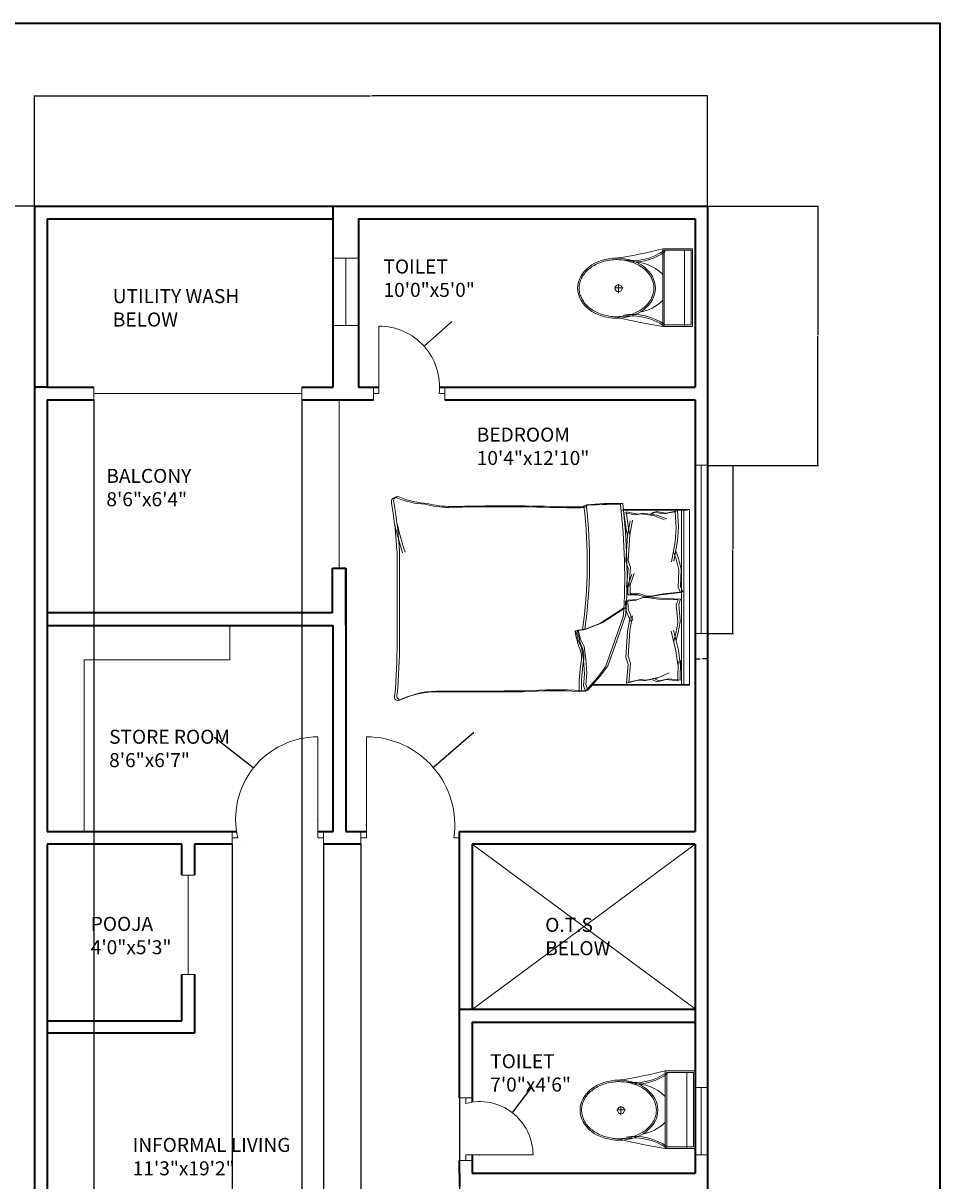
# Model space of a CAD drawing. Units: inches. Extents: x 1734 to 2405, y 1500 to 2491.
# Tile 14 of 14: x 2078 to 2405, y 2078 to 2491. Entities that reach past the tile are written whole.
import ezdxf

# ---------------------------------------------------------------- set-up
doc = ezdxf.new("R2010")
doc.units = ezdxf.units.IN
for name, color, linetype, lineweight in [('A-ANNO-DIMS', 2, 'Continuous', 18), ('A-ANNO-TTLB', 7, 'Continuous', 35), ('A-AREA-IDEN', 7, 'Continuous', 18), ('A-DOOR', 3, 'Continuous', 18), ('A-FLOR-CASE', 9, 'Continuous', 18), ('A-FLOR-FIXT', 9, 'Continuous', 18), ('A-FLOR-OPEN', 8, 'Continuous', 13), ('A-FURN', 8, 'Continuous', 13), ('A-GLAZ', 4, 'Continuous', 18), ('A-WALL', 7, 'Continuous', 35)]:
    doc.layers.add(name, color=color, linetype=linetype, lineweight=lineweight)
doc.styles.get("Standard").update_dxf_attribs({"font": 'arial.ttf'})
doc.dimstyles.get("Standard").update_dxf_attribs({"dimtxt": 0.18, "dimasz": 0.18, "dimexe": 0.18, "dimexo": 0.0625, "dimgap": 0.09, "dimtad": 0, "dimtih": 1, "dimtoh": 1, "dimdec": 4, "dimzin": 0, "dimdsep": 46, "dimtxsty": 'Standard', "dimcen": 0.09, "dimadec": 0, "dimazin": 0, "dimtfac": 1, "dimtdec": 4, "dimtofl": 0, "dimtmove": 0, "dimatfit": 3, "dimfxl": 1, "dimtolj": 1, "dimtzin": 0, "dimarcsym": 0})

# ---------------------------------------------------------------- blocks, each defined once
blk = doc.blocks.new('A$C31115884')
for p, q in [((283.1, 497.7), (223.4, 497.7)), ((257.5, 466.4), (257.5, 523.2)), ((0, 200), (0, 0)), ((520, 200), (0, 200)), ((10, 190), (10, 10)), ((510, 190), (10, 190)), ((510, 10), (510, 190)), ((520, 0), (520, 200)), ((510, 54.5), (0, 54.5)), ((10, 10), (510, 10)), ((0, 0), (520, 0))]:
    blk.add_line(p, q)
blk.add_circle((255.6, 496.4), 23.6)
for centre, radius, start, end in [((2777.7, -204.6), 2807, 165.4549, 171.71327), ((3237, 905), 2807, 188.28673, 194.5451), ((-294.5, 403.3), 364.7, 324.20913, 9.34987), ((-294.5, 403.3), 374.7, 324.20913, 9.34987), ((139.5, 406.2), 293.5, 315.84364, 2.65635), ((805.8, 403.3), 374.7, 179.20365, 215.79087), ((805.8, 403.3), 364.7, 170.65013, 215.79087), ((383.6, 406.2), 293.5, 190.27735, 224.15636)]:
    blk.add_arc(centre, radius, start, end)
blk.add_ellipse((256.2, 509.9), major_axis=(0, -260.7), ratio=0.772727)
blk.add_open_spline([(256.2, 259.2), (263.1, 259.2), (270, 259.7), (287.8, 262.3), (298.7, 265.1), (319.9, 273.1), (330.2, 278.4), (350.1, 291.1), (359.7, 298.7), (377.7, 315.9), (386.2, 325.5), (401.7, 346.6), (408.8, 358.1), (421.3, 382.5), (426.8, 395.5), (435.9, 422.4), (439.5, 436.4), (444.8, 465.1), (446.5, 479.7), (447.9, 509.2), (447.6, 524), (445, 553.3), (442.7, 567.8), (436.3, 596), (432.1, 609.7), (421.9, 636), (416, 648.6), (402.5, 672.1), (395, 683), (378.6, 703), (369.8, 712.1), (351.1, 728), (341.3, 734.8), (320.9, 746.2), (310.4, 750.7), (288.9, 757.3), (278, 759.4), (256, 761), (245, 760.6), (223.1, 757.2), (212.3, 754.3), (191.1, 746.1), (180.8, 740.7), (160.9, 727.8), (151.4, 720.1), (133.5, 702.7), (125.1, 693), (109.6, 671.7), (102.6, 660.2), (90.2, 635.7), (84.9, 622.7), (76, 595.6), (72.4, 581.6), (67.2, 552.9), (65.6, 538.2), (64.4, 508.8), (64.8, 494), (67.5, 464.7), (69.9, 450.2), (76.6, 422), (80.8, 408.3), (91.1, 382.2), (97.2, 369.7), (110.8, 346.3), (118.4, 335.4), (134.8, 315.6), (143.7, 306.7), (162.4, 290.9), (172.3, 284.2), (192.8, 273), (203.3, 268.6), (224.8, 262.2), (235.8, 260.2), (249.9, 259.3), (253, 259.2), (256.2, 259.2)], degree=3, knots=[0, 0, 0, 0, 0.110105, 0.110105, 0.285049, 0.285049, 0.459994, 0.459994, 0.634938, 0.634938, 0.809882, 0.809882, 0.984827, 0.984827, 1.159771, 1.159771, 1.334715, 1.334715, 1.50966, 1.50966, 1.684604, 1.684604, 1.859549, 1.859549, 2.034493, 2.034493, 2.209437, 2.209437, 2.384382, 2.384382, 2.559326, 2.559326, 2.73427, 2.73427, 2.909215, 2.909215, 3.084159, 3.084159, 3.259103, 3.259103, 3.434048, 3.434048, 3.608992, 3.608992, 3.783936, 3.783936, 3.958881, 3.958881, 4.133825, 4.133825, 4.30877, 4.30877, 4.483714, 4.483714, 4.658658, 4.658658, 4.833603, 4.833603, 5.008547, 5.008547, 5.183491, 5.183491, 5.358436, 5.358436, 5.53338, 5.53338, 5.708324, 5.708324, 5.883269, 5.883269, 6.058213, 6.058213, 6.233158, 6.233158, 6.283185, 6.283185, 6.283185, 6.283185])
blk = doc.blocks.new('BED-DOUBLE')
for p, q in [((81.88, 67.96), (105.53, 67.96)), ((81.88, 67.96), (105.53, 67.96)), ((82.71, 68.26), (106.37, 68.26)), ((82.71, 68.26), (106.37, 68.26)), ((83.83, 60.38), (82.88, 67.03)), ((82.88, 67.03), (87.04, 66.28)), ((83.83, 60.38), (82.88, 67.03)), ((82.88, 67.03), (87.04, 66.28)), ((84.66, 60.68), (83.72, 67.33)), ((83.72, 67.33), (87.87, 66.58)), ((84.66, 60.68), (83.72, 67.33)), ((83.72, 67.33), (87.87, 66.58)), ((87.04, 66.28), (89.12, 66.66)), ((87.04, 66.28), (89.12, 66.66)), ((87.87, 66.58), (89.95, 66.95)), ((87.87, 66.58), (89.95, 66.95)), ((89.12, 66.66), (93.84, 65.9)), ((89.12, 66.66), (93.84, 65.9)), ((89.95, 66.95), (94.67, 66.2)), ((89.95, 66.95), (94.67, 66.2)), ((93.65, 67.22), (92.33, 66.47)), ((93.65, 67.22), (92.33, 66.47)), ((94.48, 67.52), (93.16, 66.77)), ((94.48, 67.52), (93.16, 66.77)), ((97.05, 66.66), (93.65, 67.22)), ((97.05, 66.66), (93.65, 67.22)), ((97.88, 66.95), (94.48, 67.52)), ((97.88, 66.95), (94.48, 67.52)), ((94.67, 66.2), (98.26, 64.88)), ((94.67, 66.2), (98.26, 64.88)), ((101.2, 67.41), (97.05, 66.66)), ((101.2, 67.41), (97.05, 66.66)), ((102.04, 67.71), (97.88, 66.95)), ((102.04, 67.71), (97.88, 66.95)), ((101.17, 67.41), (101.6, 61.81)), ((101.17, 67.41), (101.6, 61.82)), ((102.01, 67.7), (102.44, 62.11)), ((102.01, 67.7), (102.44, 62.11)), ((103.53, 67.96), (103.53, 5.54)), ((103.53, 67.96), (103.53, 5.54)), ((104.36, 68.26), (104.36, 5.84)), ((104.36, 68.26), (104.36, 5.84)), ((106.37, 5.54), (106.37, 67.96)), ((85.12, 64.16), (84.25, 58.9)), ((85.12, 64.16), (84.25, 58.9)), ((85.96, 64.46), (85.09, 59.2)), ((85.96, 64.46), (85.09, 59.2)), ((93.84, 65.9), (97.42, 64.58)), ((93.84, 65.9), (97.42, 64.58)), ((102.41, 61.98), (102.04, 56.98)), ((102.41, 61.98), (102.04, 56.98)), ((102.44, 62.11), (102.41, 61.98)), ((102.44, 62.11), (102.41, 61.98)), ((84.25, 58.9), (83.69, 49.74)), ((84.25, 58.9), (83.69, 49.74)), ((84.25, 58.9), (83.83, 60.38)), ((84.25, 58.9), (83.83, 60.38)), ((85.09, 59.2), (84.52, 50.04)), ((85.09, 59.2), (84.52, 50.04)), ((85.09, 59.2), (84.66, 60.68)), ((85.09, 59.2), (84.66, 60.68)), ((101.58, 61.68), (101.2, 56.68)), ((101.58, 61.68), (101.2, 56.68)), ((101.6, 61.82), (101.58, 61.68)), ((101.6, 61.81), (101.58, 61.68)), ((101.2, 56.68), (99.88, 49.51)), ((101.2, 56.68), (99.88, 49.51)), ((102.04, 56.98), (100.71, 49.81)), ((102.04, 56.98), (100.71, 49.81)), ((2.04, 52.82), (2.04, 20.68)), ((2.04, 52.82), (2.04, 20.68)), ((2.87, 53.12), (2.87, 20.98)), ((2.87, 53.12), (2.87, 20.98)), ((83.69, 49.74), (84.42, 47.18)), ((83.69, 49.74), (84.42, 47.18)), ((84.52, 50.04), (85.25, 47.48)), ((84.52, 50.04), (85.25, 47.48)), ((100.64, 53.1), (101.58, 50.45)), ((100.64, 53.1), (101.58, 50.45)), ((101.47, 53.4), (102.41, 50.75)), ((101.47, 53.39), (102.41, 50.75)), ((101.58, 50.45), (102.52, 46.68)), ((101.58, 50.45), (102.52, 46.68)), ((102.41, 50.75), (103.36, 46.98)), ((102.41, 50.75), (103.36, 46.98)), ((84.42, 47.18), (83.89, 40.48)), ((84.42, 47.18), (83.89, 40.48)), ((85.25, 47.48), (84.72, 40.78)), ((85.25, 47.48), (84.72, 40.78)), ((85.13, 41.32), (86.55, 45.42)), ((85.13, 41.32), (86.55, 45.42)), ((102.52, 46.26), (102.33, 40.45)), ((102.52, 46.26), (102.33, 40.45)), ((102.52, 46.68), (102.52, 46.26)), ((102.52, 46.68), (102.52, 46.26)), ((103.36, 46.56), (103.17, 40.75)), ((103.36, 46.56), (103.17, 40.75)), ((103.36, 46.98), (103.36, 46.56)), ((103.36, 46.98), (103.36, 46.56)), ((84.29, 41.02), (85.72, 45.13)), ((84.29, 41.02), (85.72, 45.12)), ((85.13, 38.11), (85.13, 41.32)), ((85.13, 38.11), (85.13, 41.32)), ((84.29, 37.81), (84.29, 41.02)), ((84.29, 37.81), (84.29, 41.02)), ((87.79, 37.81), (84.29, 37.81)), ((87.79, 37.81), (84.29, 37.81)), ((88.63, 38.11), (85.13, 38.11)), ((88.63, 38.11), (85.13, 38.11)), ((90.25, 37.05), (87.79, 37.81)), ((90.25, 37.05), (87.79, 37.81)), ((91.08, 37.35), (88.63, 38.11)), ((91.08, 37.35), (88.63, 38.11)), ((92.78, 37.35), (91.08, 37.35)), ((92.78, 37.35), (91.08, 37.35)), ((96.1, 37.81), (91.95, 37.05)), ((96.1, 37.81), (91.95, 37.05)), ((96.94, 38.11), (92.78, 37.35)), ((96.94, 38.11), (92.78, 37.35)), ((103.09, 38.56), (96.1, 37.81)), ((103.09, 38.56), (96.1, 37.81)), ((103.92, 38.86), (96.94, 38.11)), ((103.92, 38.86), (96.94, 38.11)), ((102.33, 40.45), (103.09, 38.56)), ((102.33, 40.45), (103.09, 38.56)), ((103.17, 40.75), (103.92, 38.86)), ((103.17, 40.75), (103.92, 38.86)), ((83.66, 33.28), (75.18, 27.8)), ((83.66, 33.28), (75.18, 27.8)), ((86.97, 35.76), (83.47, 35.54)), ((86.97, 35.76), (83.47, 35.54)), ((83.47, 35.54), (83.67, 32.34)), ((83.47, 35.54), (83.67, 32.34)), ((87.8, 36.06), (84.3, 35.84)), ((87.8, 36.06), (84.3, 35.84)), ((84.3, 35.84), (84.51, 32.63)), ((84.3, 35.84), (84.51, 32.64)), ((89.37, 36.67), (86.97, 35.76)), ((89.37, 36.67), (86.97, 35.76)), ((90.2, 36.96), (87.8, 36.06)), ((90.2, 36.96), (87.8, 36.06)), ((91.06, 36.77), (89.37, 36.67)), ((91.06, 36.77), (89.37, 36.67)), ((91.9, 37.07), (90.2, 36.96)), ((91.9, 37.07), (90.2, 36.96)), ((91.95, 37.05), (90.25, 37.05)), ((91.95, 37.05), (90.25, 37.05)), ((95.26, 36.28), (91.06, 36.77)), ((95.26, 36.28), (91.06, 36.77)), ((96.09, 36.57), (91.9, 37.07)), ((96.09, 36.58), (91.9, 37.07)), ((102.28, 35.96), (95.26, 36.28)), ((102.28, 35.96), (95.26, 36.28)), ((103.11, 36.26), (96.09, 36.58)), ((103.11, 36.26), (96.09, 36.57)), ((101.64, 34.03), (102.28, 35.96)), ((101.64, 34.03), (102.28, 35.96)), ((102.19, 28.24), (101.64, 34.03)), ((102.19, 28.24), (101.64, 34.03)), ((102.48, 34.33), (103.11, 36.26)), ((102.48, 34.33), (103.11, 36.26)), ((103.03, 28.54), (102.48, 34.33)), ((103.03, 28.54), (102.48, 34.33)), ((82.83, 32.98), (74.35, 27.51)), ((82.83, 32.98), (74.35, 27.51)), ((79, 19.42), (82.83, 30.31)), ((79, 19.41), (82.83, 30.3)), ((79.83, 19.71), (83.66, 30.6)), ((79.83, 19.71), (83.66, 30.6)), ((83.67, 32.34), (85.35, 28.33)), ((83.67, 32.34), (85.35, 28.33)), ((85.12, 29.97), (84.25, 24.7)), ((85.12, 29.97), (84.25, 24.7)), ((84.51, 32.64), (86.18, 28.63)), ((84.51, 32.63), (86.18, 28.62)), ((85.96, 30.27), (85.09, 25)), ((85.96, 30.27), (85.09, 25)), ((68.49, 25.28), (65.86, 24.88)), ((68.49, 25.28), (65.86, 24.88)), ((65.86, 24.88), (66.67, 21.64)), ((65.86, 24.88), (66.67, 21.64)), ((69.32, 25.58), (66.69, 25.17)), ((69.32, 25.58), (66.69, 25.17)), ((66.69, 25.17), (67.5, 21.94)), ((66.69, 25.17), (67.5, 21.94)), ((74.35, 27.51), (68.49, 25.28)), ((74.35, 27.51), (68.49, 25.28)), ((75.18, 27.8), (69.32, 25.58)), ((75.18, 27.8), (69.32, 25.58)), ((85.09, 25), (84.52, 15.84)), ((85.09, 25), (84.52, 15.85)), ((101.52, 17.76), (99.76, 24.83)), ((101.52, 17.76), (99.76, 24.83)), ((102.36, 18.05), (100.59, 25.13)), ((102.36, 18.05), (100.59, 25.13)), ((101.51, 24), (102.22, 27.83)), ((101.51, 24), (102.22, 27.83)), ((102.22, 27.83), (102.19, 28.24)), ((102.22, 27.83), (102.19, 28.24)), ((102.35, 24.3), (103.05, 28.12)), ((102.35, 24.3), (103.05, 28.12)), ((103.05, 28.12), (103.03, 28.54)), ((103.05, 28.12), (103.03, 28.54)), ((66.67, 21.64), (67.88, 19.01)), ((66.67, 21.64), (67.88, 19.01)), ((67.5, 21.94), (68.72, 19.31)), ((67.5, 21.94), (68.72, 19.31)), ((84.25, 24.7), (83.69, 15.55)), ((84.25, 24.7), (83.69, 15.55)), ((100.73, 21.3), (101.51, 24)), ((100.73, 21.3), (101.51, 24)), ((101.57, 21.6), (102.35, 24.3)), ((101.57, 21.6), (102.35, 24.3)), ((67.88, 19.01), (68.49, 14.56)), ((67.88, 19.01), (68.49, 14.56)), ((68.72, 19.31), (69.32, 14.86)), ((68.72, 19.31), (69.32, 14.86)), ((76.37, 12.13), (79, 19.42)), ((76.37, 12.13), (79, 19.41)), ((77.21, 12.43), (79.83, 19.71)), ((77.21, 12.43), (79.83, 19.71)), ((102.21, 12.8), (101.52, 17.76)), ((102.21, 12.8), (101.52, 17.76)), ((103.05, 13.09), (102.36, 18.05)), ((103.05, 13.09), (102.36, 18.05)), ((68.49, 14.56), (68.89, 9.5)), ((68.49, 14.56), (68.89, 9.5)), ((69.32, 14.86), (69.73, 9.8)), ((69.32, 14.86), (69.73, 9.8)), ((74.38, 8.59), (77.21, 12.43)), ((74.38, 8.59), (77.21, 12.43)), ((83.69, 15.55), (84.42, 12.99)), ((83.69, 15.55), (84.42, 12.99)), ((84.42, 12.99), (83.89, 6.28)), ((84.42, 12.99), (83.89, 6.28)), ((84.52, 15.85), (85.25, 13.28)), ((84.52, 15.84), (85.25, 13.28)), ((85.25, 13.28), (84.72, 6.58)), ((85.25, 13.28), (84.72, 6.58)), ((102.19, 7.05), (102.32, 14.11)), ((102.19, 7.05), (102.32, 14.11)), ((102.32, 14.11), (102.21, 12.8)), ((102.32, 14.11), (102.21, 12.8)), ((103.03, 7.35), (103.15, 14.4)), ((103.03, 7.35), (103.15, 14.4)), ((103.15, 14.4), (103.05, 13.09)), ((103.15, 14.4), (103.05, 13.09)), ((68.89, 9.5), (68.49, 5.46)), ((68.89, 9.5), (68.49, 5.46)), ((69.3, 3.45), (73.54, 8.29)), ((69.3, 3.45), (73.54, 8.29)), ((69.73, 9.8), (69.32, 5.76)), ((69.73, 9.8), (69.32, 5.76)), ((70.13, 3.75), (74.38, 8.59)), ((70.13, 3.75), (74.38, 8.59)), ((73.54, 8.29), (76.37, 12.13)), ((73.54, 8.29), (76.37, 12.13)), ((90.92, 7.35), (95.58, 8.4)), ((90.92, 7.35), (95.58, 8.4)), ((94.75, 8.1), (98.25, 9.64)), ((94.75, 8.1), (98.25, 9.64)), ((95.58, 8.4), (99.08, 9.94)), ((95.58, 8.4), (99.08, 9.94)), ((68.49, 5.46), (69.3, 3.45)), ((68.49, 5.46), (69.3, 3.45)), ((69.32, 5.76), (70.13, 3.75)), ((69.32, 5.76), (70.13, 3.75)), ((105.53, 5.54), (70.78, 5.54)), ((105.53, 5.54), (70.78, 5.54)), ((106.37, 5.84), (71.61, 5.84)), ((106.37, 5.84), (71.61, 5.84)), ((83.89, 6.28), (87.99, 7.3)), ((83.89, 6.28), (87.99, 7.3)), ((84.72, 6.58), (88.82, 7.6)), ((84.72, 6.58), (88.82, 7.59)), ((87.99, 7.3), (90.08, 7.05)), ((87.99, 7.3), (90.08, 7.05)), ((88.82, 7.6), (90.92, 7.35)), ((88.82, 7.59), (90.92, 7.35)), ((90.08, 7.05), (94.75, 8.1)), ((90.08, 7.05), (94.75, 8.1)), ((94.64, 6.77), (93.28, 7.44)), ((94.64, 6.77), (93.28, 7.44)), ((95.48, 7.07), (94.11, 7.74)), ((95.48, 7.07), (94.11, 7.74)), ((98, 7.54), (94.64, 6.77)), ((98, 7.54), (94.64, 6.77)), ((98.83, 7.84), (95.48, 7.07)), ((98.83, 7.84), (95.48, 7.07)), ((102.19, 7.05), (98, 7.54)), ((102.19, 7.05), (98, 7.54)), ((103.03, 7.35), (98.83, 7.84)), ((103.03, 7.35), (98.83, 7.84)), ((106.37, 5.54), (105.53, 5.54)), ((67.02, 3.35), (69.3, 3.45, 5.06)), ((67.02, 3.35), (69.3, 3.45, 5.06)), ((67.85, 3.65), (70.13, 3.75, 5.06)), ((67.85, 3.65), (70.13, 3.75, 5.06))]:
    blk.add_line(p, q)
for centre, radius, start, end in [((1.42, 71.08), 1.42, 56.1736, 203.4781), ((1.42, 71.08), 1.42, 56.1736, 203.4781), ((-156.77, 44.51), 159.02, 2.9958, 9.4091), ((-156.77, 44.51), 159.02, 2.9958, 9.4091), ((2.25, 71.38), 1.42, 56.1736, 203.4781), ((2.25, 71.38), 1.42, 56.1736, 203.4781), ((-155.93, 44.81), 159.02, 2.9958, 9.4091), ((-155.93, 44.81), 159.02, 2.9958, 9.4091), ((13.75, 100.79), 30.77, 247.9751, 266.652), ((13.75, 100.79), 30.77, 247.9751, 266.652), ((14.58, 101.08), 30.77, 247.9751, 266.652), ((14.58, 101.08), 30.77, 247.9751, 266.652), ((22.11, 107.93), 38.7, 256.0648, 268.9113), ((22.11, 107.93), 38.7, 256.0648, 268.9113), ((80.12, -38.43), 108.8, 88.7218, 95.604), ((80.12, -38.43), 108.8, 88.7218, 95.604), ((-131.4, 44.9), 215.46, 356.0865, 6.7821), ((-131.4, 44.9), 215.46, 356.0865, 6.7821), ((21.27, 107.63), 38.7, 256.0648, 268.9113), ((21.27, 107.63), 38.7, 256.0648, 268.9113), ((39.43, -560.7), 629.91, 88.22771, 91.71854), ((39.43, -560.7), 629.91, 88.22771, 91.71854), ((40.26, -560.4), 629.91, 88.22771, 91.71854), ((40.26, -560.4), 629.91, 88.22771, 91.71854), ((64.82, 291.01), 222.17, 268.4762, 271.0082), ((64.82, 291.01), 222.17, 268.4762, 271.0082), ((65.65, 291.31), 222.17, 268.4762, 271.0082), ((65.65, 291.31), 222.17, 268.4762, 271.0082), ((-98.62, 49.31), 168.5, 351.7845, 6.9006), ((-98.62, 49.31), 168.5, 351.7845, 6.9006), ((79.29, -38.73), 108.8, 88.7218, 95.604), ((79.29, -38.73), 108.8, 88.7218, 95.604), ((-97.79, 49.61), 168.5, 351.7845, 6.9006), ((-97.79, 49.61), 168.5, 351.7845, 6.9006), ((-132.23, 44.6), 215.46, 356.0865, 6.7821), ((-132.23, 44.6), 215.46, 356.0865, 6.7821), ((136.5, 94.99), 139.04, 193.3832, 197.7053), ((136.5, 94.99), 139.04, 193.3832, 197.7053), ((137.34, 95.29), 139.04, 193.3832, 197.7053), ((137.34, 95.29), 139.04, 193.3832, 197.7053), ((65.78, 24.65), 0.241, 70.2464, 181.1377), ((65.78, 24.65), 0.241, 70.2464, 181.1377), ((66.61, 24.95), 0.241, 70.2464, 181.1377), ((66.61, 24.95), 0.241, 70.2464, 181.1377), ((104.43, 32.11), 38.73, 190.6617, 199.8806), ((104.43, 32.11), 38.73, 190.6617, 199.8806), ((-171.71, 18.75), 173.75, 354.4998, 0.6351), ((-171.71, 18.75), 173.75, 354.4998, 0.6351), ((-170.87, 19.05), 173.75, 354.4998, 0.6351), ((-170.87, 19.05), 173.75, 354.4998, 0.6351), ((103.6, 31.81), 38.73, 190.6617, 199.8806), ((103.6, 31.81), 38.73, 190.6617, 199.8806), ((59.73, 15.37), 8.13, 348.6608, 23.7384), ((59.73, 15.37), 8.13, 348.6608, 23.7384), ((60.57, 15.67), 8.13, 348.6608, 23.7384), ((60.57, 15.67), 8.13, 348.6608, 23.7384), ((114.23, 5.46), 47.26, 169.8763, 182.5657), ((114.23, 5.46), 47.26, 169.8763, 182.5657), ((115.06, 5.76), 47.26, 169.8763, 182.5657), ((115.06, 5.76), 47.26, 169.8763, 182.5657), ((2.53, 1.44), 1.44, 152.6588, 266.02), ((2.53, 1.44), 1.44, 152.6588, 266.02), ((3.36, 1.73), 1.44, 152.6588, 266.02), ((3.36, 1.74), 1.44, 152.6588, 266.02), ((15.85, -26.97), 30.12, 87.4714, 116.4681), ((15.85, -26.97), 30.12, 87.4714, 116.4681), ((16.69, -26.67), 30.12, 87.4714, 116.4681), ((16.69, -26.67), 30.12, 87.4714, 116.4681), ((16.96, 5961.08), 5957.95, 270.002168, 270.286887), ((16.96, 5961.08), 5957.95, 270.002168, 270.286887), ((17.79, 5961.38), 5957.95, 270.002168, 270.286887), ((17.79, 5961.38), 5957.95, 270.002168, 270.286887), ((58.1, -165.55), 169.13, 86.9791, 93.8365), ((58.1, -165.55), 169.13, 86.9791, 93.8365), ((58.94, -165.25), 169.13, 86.9791, 93.8365), ((58.94, -165.25), 169.13, 86.9791, 93.8365)]:
    blk.add_arc(centre, radius, start, end)
blk = doc.blocks.new('WIN-60')
for p, q in [((0, 60), (4.5, 60)), ((4.5, 60), (2.25, 60)), ((2.25, 60), (2.25, 0)), ((2.25, 0), (0, 0)), ((0, 0), (4.5, 0))]:
    blk.add_line(p, q)
blk = doc.blocks.new('*D20')
at = {"layer": 'A-ANNO-DIMS', "color": 0, "lineweight": -2, "transparency": 16777216}
for p, q in [((2321.81, 2333.41), (2330.92, 2333.41)), ((2330.74, 2333.23), (2330.74, 2303.6)), ((2330.74, 2273.59), (2330.74, 2303.23)), ((2321.81, 2273.41), (2330.92, 2273.41))]:
    blk.add_line(p, q, dxfattribs=at)
at = {"layer": 'A-ANNO-DIMS', "color": 0, "transparency": 16777216}
for points in [[(2330.71, 2333.23), (2330.77, 2333.23), (2330.74, 2333.41)], [(2330.71, 2273.59), (2330.77, 2273.59), (2330.74, 2273.41)]]:
    blk.add_solid(points, dxfattribs=at)
at = {"layer": 'Defpoints', "color": 0, "transparency": 16777216}
for p in [(2321.74, 2333.41), (2330.74, 2333.41), (2321.74, 2273.41)]:
    blk.add_point(p, dxfattribs=at)
at = {"layer": 'A-ANNO-DIMS', "color": 0, "transparency": 16777216, "insert": (2330.74, 2303.41), "char_height": 0.18, "attachment_point": 5}
blk.add_mtext('\\A1;WINDOW 60 TYP.', dxfattribs=at)
blk = doc.blocks.new('*D21')
at = {"layer": 'A-ANNO-DIMS', "color": 0, "lineweight": -2, "transparency": 16777216}
for p, q in [((2317.24, 2273.35), (2317.24, 2264.23)), ((2321.74, 2273.35), (2321.74, 2264.23)), ((2317.42, 2264.41), (2319.04, 2264.41)), ((2321.56, 2264.41), (2319.95, 2264.41))]:
    blk.add_line(p, q, dxfattribs=at)
at = {"layer": 'A-ANNO-DIMS', "color": 0, "transparency": 16777216}
for points in [[(2317.42, 2264.44), (2317.42, 2264.38), (2317.24, 2264.41)], [(2321.56, 2264.44), (2321.56, 2264.38), (2321.74, 2264.41)]]:
    blk.add_solid(points, dxfattribs=at)
at = {"layer": 'Defpoints', "color": 0, "transparency": 16777216}
for p in [(2317.24, 2273.41), (2321.74, 2273.41), (2321.74, 2264.41)]:
    blk.add_point(p, dxfattribs=at)
at = {"layer": 'A-ANNO-DIMS', "color": 0, "transparency": 16777216, "insert": (2319.49, 2264.41), "char_height": 0.18, "attachment_point": 5}
blk.add_mtext('\\A1;5 TYP.', dxfattribs=at)
blk = doc.blocks.new('*D35')
at = {"layer": 'A-ANNO-DIMS', "color": 0, "lineweight": -2, "transparency": 16777216}
for p, q in [((2081.74, 2425.89), (2081.74, 2465.35)), ((2081.92, 2465.17), (2201.45, 2465.17)), ((2321.56, 2465.17), (2202.03, 2465.17)), ((2321.74, 2425.89), (2321.74, 2465.35))]:
    blk.add_line(p, q, dxfattribs=at)
at = {"layer": 'A-ANNO-DIMS', "color": 0, "transparency": 16777216}
for points in [[(2081.92, 2465.2), (2081.92, 2465.14), (2081.74, 2465.17)], [(2321.56, 2465.2), (2321.56, 2465.14), (2321.74, 2465.17)]]:
    blk.add_solid(points, dxfattribs=at)
at = {"layer": 'Defpoints', "color": 0, "transparency": 16777216}
for p in [(2321.74, 2465.17), (2081.74, 2425.82), (2321.74, 2425.82)]:
    blk.add_point(p, dxfattribs=at)
at = {"layer": 'A-ANNO-DIMS', "color": 0, "transparency": 16777216, "insert": (2201.74, 2465.17), "char_height": 0.18, "attachment_point": 5}
blk.add_mtext('\\A1;240', dxfattribs=at)
blk = doc.blocks.new('*D36')
at = {"layer": 'A-ANNO-DIMS', "color": 0, "lineweight": -2, "transparency": 16777216}
for p, q in [((2081.68, 2425.82), (2042.21, 2425.82)), ((2042.39, 2425.64), (2042.39, 2065.96)), ((2042.39, 1705.92), (2042.39, 2065.6)), ((2081.68, 1705.74), (2042.21, 1705.74))]:
    blk.add_line(p, q, dxfattribs=at)
at = {"layer": 'A-ANNO-DIMS', "color": 0, "transparency": 16777216}
for points in [[(2042.36, 2425.64), (2042.42, 2425.64), (2042.39, 2425.82)], [(2042.36, 1705.92), (2042.42, 1705.92), (2042.39, 1705.74)]]:
    blk.add_solid(points, dxfattribs=at)
at = {"layer": 'Defpoints', "color": 0, "transparency": 16777216}
for p in [(2042.39, 2425.82), (2081.74, 2425.82), (2081.74, 1705.74)]:
    blk.add_point(p, dxfattribs=at)
at = {"layer": 'A-ANNO-DIMS', "color": 0, "transparency": 16777216, "insert": (2042.39, 2065.78), "char_height": 0.18, "attachment_point": 5}
blk.add_mtext('\\A1;720.1', dxfattribs=at)
blk = doc.blocks.new('*D40')
at = {"layer": 'A-ANNO-DIMS', "color": 0, "lineweight": -2, "transparency": 16777216}
for p, q in [((2321.81, 2425.82), (2361.27, 2425.82)), ((2361.09, 2425.64), (2361.09, 2379.8)), ((2361.09, 2333.59), (2361.09, 2379.44)), ((2321.81, 2333.41), (2361.27, 2333.41))]:
    blk.add_line(p, q, dxfattribs=at)
at = {"layer": 'A-ANNO-DIMS', "color": 0, "transparency": 16777216}
for points in [[(2361.06, 2425.64), (2361.12, 2425.64), (2361.09, 2425.82)], [(2361.06, 2333.59), (2361.12, 2333.59), (2361.09, 2333.41)]]:
    blk.add_solid(points, dxfattribs=at)
at = {"layer": 'Defpoints', "color": 0, "transparency": 16777216}
for p in [(2321.74, 2425.82), (2361.09, 2425.82), (2321.74, 2333.41)]:
    blk.add_point(p, dxfattribs=at)
at = {"layer": 'A-ANNO-DIMS', "color": 0, "transparency": 16777216, "insert": (2361.09, 2379.62), "char_height": 0.18, "attachment_point": 5}
blk.add_mtext('\\A1;92.41', dxfattribs=at)
blk = doc.blocks.new('*D42')
at = {"layer": 'A-ANNO-DIMS', "color": 0, "lineweight": -2, "transparency": 16777216}
for p, q in [((2152.2, 2198.26), (2152.2, 1611.24)), ((2184.72, 2198.26), (2184.72, 1611.24)), ((2152.38, 1611.42), (2168, 1611.42)), ((2184.54, 1611.42), (2168.92, 1611.42))]:
    blk.add_line(p, q, dxfattribs=at)
at = {"layer": 'A-ANNO-DIMS', "color": 0, "transparency": 16777216}
for points in [[(2152.38, 1611.45), (2152.38, 1611.39), (2152.2, 1611.42)], [(2184.54, 1611.45), (2184.54, 1611.39), (2184.72, 1611.42)]]:
    blk.add_solid(points, dxfattribs=at)
at = {"layer": 'Defpoints', "color": 0, "transparency": 16777216}
for p in [(2152.2, 2198.32), (2184.72, 2198.32), (2184.72, 1611.42)]:
    blk.add_point(p, dxfattribs=at)
at = {"layer": 'A-ANNO-DIMS', "color": 0, "transparency": 16777216, "insert": (2168.46, 1611.42), "char_height": 0.18, "attachment_point": 5}
blk.add_mtext('\\A1;32.526', dxfattribs=at)
blk = doc.blocks.new('*D43')
at = {"layer": 'A-ANNO-DIMS', "color": 0, "lineweight": -2, "transparency": 16777216}
for p, q in [((2198.08, 2198.26), (2198.08, 1611.24)), ((2233.24, 2200.45), (2233.24, 1611.24)), ((2198.26, 1611.42), (2215.27, 1611.42)), ((2233.06, 1611.42), (2216.05, 1611.42))]:
    blk.add_line(p, q, dxfattribs=at)
at = {"layer": 'A-ANNO-DIMS', "color": 0, "transparency": 16777216}
for points in [[(2198.26, 1611.45), (2198.26, 1611.39), (2198.08, 1611.42)], [(2233.06, 1611.45), (2233.06, 1611.39), (2233.24, 1611.42)]]:
    blk.add_solid(points, dxfattribs=at)
at = {"layer": 'Defpoints', "color": 0, "transparency": 16777216}
for p in [(2198.08, 2198.32), (2233.24, 2200.51), (2233.24, 1611.42)]:
    blk.add_point(p, dxfattribs=at)
at = {"layer": 'A-ANNO-DIMS', "color": 0, "transparency": 16777216, "insert": (2215.66, 1611.42), "char_height": 0.18, "attachment_point": 5}
blk.add_mtext('\\A1;35.17', dxfattribs=at)
blk = doc.blocks.new('*D44')
at = {"layer": 'A-ANNO-DIMS', "color": 0, "lineweight": -2, "transparency": 16777216}
for p, q in [((2102.87, 2356.76), (2102.87, 1611.24)), ((2177.04, 2356.76), (2177.04, 1611.24)), ((2103.05, 1611.42), (2139.56, 1611.42)), ((2176.86, 1611.42), (2140.35, 1611.42))]:
    blk.add_line(p, q, dxfattribs=at)
at = {"layer": 'A-ANNO-DIMS', "color": 0, "transparency": 16777216}
for points in [[(2103.05, 1611.45), (2103.05, 1611.39), (2102.87, 1611.42)], [(2176.86, 1611.45), (2176.86, 1611.39), (2177.04, 1611.42)]]:
    blk.add_solid(points, dxfattribs=at)
at = {"layer": 'Defpoints', "color": 0, "transparency": 16777216}
for p in [(2102.87, 2356.82), (2177.04, 2356.82), (2177.04, 1611.42)]:
    blk.add_point(p, dxfattribs=at)
at = {"layer": 'A-ANNO-DIMS', "color": 0, "transparency": 16777216, "insert": (2139.96, 1611.42), "char_height": 0.18, "attachment_point": 5}
blk.add_mtext('\\A1;74.17', dxfattribs=at)
blk = doc.blocks.new('*D51')
at = {"layer": 'A-ANNO-DIMS', "color": 0, "lineweight": -2, "transparency": 16777216}
for p, q in [((2258.97, 2111.63), (2252.14, 2102.71)), ((2259.15, 2111.63), (2258.97, 2111.63)), ((2240.37, 2087.45), (2240.55, 2087.45)), ((2240.46, 2087.36), (2240.46, 2087.54))]:
    blk.add_line(p, q, dxfattribs=at)
at = {"layer": 'A-ANNO-DIMS', "color": 0, "transparency": 16777216}
blk.add_solid([(2252.12, 2102.73), (2252.16, 2102.69), (2252.03, 2102.57)], dxfattribs=at)
at = {"layer": 'Defpoints', "color": 0, "transparency": 16777216}
for p in [(2252.03, 2102.57), (2240.46, 2087.45)]:
    blk.add_point(p, dxfattribs=at)
at = {"layer": 'A-ANNO-DIMS', "color": 0, "transparency": 16777216, "insert": (2259.63, 2111.63), "char_height": 0.18, "attachment_point": 5}
blk.add_mtext('\\A1;R19.03', dxfattribs=at)
blk = doc.blocks.new('*D52')
at = {"layer": 'A-ANNO-DIMS', "color": 0, "lineweight": -2, "transparency": 16777216}
for p, q in [((2238.21, 2238.03), (2224.05, 2225.79)), ((2238.39, 2238.03), (2238.21, 2238.03)), ((2199.99, 2205.08), (2200.17, 2205.08)), ((2200.08, 2204.99), (2200.08, 2205.17))]:
    blk.add_line(p, q, dxfattribs=at)
at = {"layer": 'A-ANNO-DIMS', "color": 0, "transparency": 16777216}
blk.add_solid([(2224.03, 2225.81), (2224.07, 2225.77), (2223.91, 2225.67)], dxfattribs=at)
at = {"layer": 'Defpoints', "color": 0, "transparency": 16777216}
for p in [(2223.91, 2225.67), (2200.08, 2205.08)]:
    blk.add_point(p, dxfattribs=at)
at = {"layer": 'A-ANNO-DIMS', "color": 0, "transparency": 16777216, "insert": (2238.8, 2238.03), "char_height": 0.18, "attachment_point": 5}
blk.add_mtext('\\A1;R31.5', dxfattribs=at)
blk = doc.blocks.new('*D53')
at = {"layer": 'A-ANNO-DIMS', "color": 0, "lineweight": -2, "transparency": 16777216}
for p, q in [((2145.8, 2236.39), (2145.98, 2236.39)), ((2145.98, 2236.39), (2159.62, 2225.58)), ((2182.63, 2207.27), (2182.81, 2207.27)), ((2182.72, 2207.18), (2182.72, 2207.36))]:
    blk.add_line(p, q, dxfattribs=at)
at = {"layer": 'A-ANNO-DIMS', "color": 0, "transparency": 16777216}
blk.add_solid([(2159.64, 2225.61), (2159.6, 2225.56), (2159.76, 2225.47)], dxfattribs=at)
at = {"layer": 'Defpoints', "color": 0, "transparency": 16777216}
for p in [(2159.76, 2225.47), (2182.72, 2207.27)]:
    blk.add_point(p, dxfattribs=at)
at = {"layer": 'A-ANNO-DIMS', "color": 0, "transparency": 16777216, "insert": (2145.39, 2236.39), "char_height": 0.18, "attachment_point": 5}
blk.add_mtext('\\A1;R29.3', dxfattribs=at)
blk = doc.blocks.new('*D54')
at = {"layer": 'A-ANNO-DIMS', "color": 0, "lineweight": -2, "transparency": 16777216}
for p, q in [((2230.29, 2384.51), (2220.77, 2375.99)), ((2230.47, 2384.51), (2230.29, 2384.51)), ((2204.45, 2361.49), (2204.63, 2361.49)), ((2204.54, 2361.4), (2204.54, 2361.58))]:
    blk.add_line(p, q, dxfattribs=at)
at = {"layer": 'A-ANNO-DIMS', "color": 0, "transparency": 16777216}
blk.add_solid([(2220.75, 2376.02), (2220.79, 2375.97), (2220.64, 2375.87)], dxfattribs=at)
at = {"layer": 'Defpoints', "color": 0, "transparency": 16777216}
for p in [(2220.64, 2375.87), (2204.54, 2361.49)]:
    blk.add_point(p, dxfattribs=at)
at = {"layer": 'A-ANNO-DIMS', "color": 0, "transparency": 16777216, "insert": (2231.02, 2384.51), "char_height": 0.18, "attachment_point": 5}
blk.add_mtext('\\A1;R21.588', dxfattribs=at)

msp = doc.modelspace()

# ---------------------------------------------------------------- linework, layer by layer
at = {"layer": 'A-ANNO-TTLB'}
msp.add_lwpolyline([(1734.1307, 2491.1293), (2404.5589, 2491.1293), (2404.5589, 1500.293), (1734.1307, 1500.293)], close=True, dxfattribs=at)
at = {"layer": 'A-DOOR'}
for p, q in [((2204.5405, 2359.0746), (2204.5405, 2383.0746)), ((2202.5405, 2361.3246), (2202.5405, 2356.8246)), ((2202.5405, 2356.8246), (2202.5405, 2359.0746)), ((2202.5405, 2359.0746), (2204.5405, 2359.0746)), ((2227.9931, 2359.0746), (2225.9931, 2359.0746)), ((2227.9931, 2361.3246), (2227.9931, 2356.8246)), ((2227.9931, 2356.8246), (2227.9931, 2359.0746)), ((2182.7241, 2200.5746), (2182.7241, 2236.5746)), ((2200.0776, 2200.5746), (2200.0776, 2236.5746)), ((2152.1978, 2202.8246), (2152.1978, 2198.3246)), ((2184.7241, 2202.8246), (2184.7241, 2198.3246)), ((2198.0776, 2202.8246), (2198.0776, 2198.3246)), ((2152.1978, 2198.3246), (2152.1978, 2200.5746)), ((2152.1978, 2200.5746), (2154.1978, 2200.5746)), ((2184.7241, 2200.5746), (2182.7241, 2200.5746)), ((2184.7241, 2198.3246), (2184.7241, 2200.5746)), ((2198.0776, 2198.3246), (2198.0776, 2200.5746)), ((2198.0776, 2200.5746), (2200.0776, 2200.5746)), ((2233.2445, 2200.5102), (2231.2445, 2200.5102)), ((2237.7445, 2107.8246), (2233.2445, 2107.8246)), ((2233.2445, 2107.8246), (2235.4945, 2107.8246)), ((2235.4945, 2107.8246), (2235.4945, 2105.8246)), ((2237.7445, 2085.4536), (2233.2445, 2085.4536)), ((2233.2445, 2085.4536), (2235.4945, 2085.4536)), ((2235.4945, 2085.4536), (2235.4945, 2087.4536)), ((2235.4945, 2087.4536), (2259.4945, 2087.4536))]:
    msp.add_line(p, q, dxfattribs=at)
for centre, radius, start, end in [((2204.5405, 2361.4867), 21.5878, 353.584471, 90), ((2182.7241, 2207.2724), 29.3021, 90, 193.213524), ((2200.0776, 2205.0752), 31.4994, 351.667289, 90), ((2240.4634, 2087.4536), 19.0311, 0, 105.135083)]:
    msp.add_arc(centre, radius, start, end, dxfattribs=at)
at = {"layer": 'A-FLOR-CASE'}
for p, q in [((2151.3728, 2264.0643), (2151.3728, 2276.3246)), ((2099.4028, 2202.8246), (2099.4028, 2264.0643)), ((2099.4028, 2264.0643), (2151.3728, 2264.0643))]:
    msp.add_line(p, q, dxfattribs=at)
at = {"layer": 'A-FLOR-OPEN'}
for p, q in [((2237.7445, 2198.3246), (2317.2445, 2139.5746)), ((2317.2445, 2198.3246), (2237.7445, 2139.3246))]:
    msp.add_line(p, q, dxfattribs=at)
at = {"layer": 'A-GLAZ'}
for p, q in [((2188.2445, 2407.2516), (2197.2445, 2407.2516)), ((2197.2445, 2407.2516), (2192.7445, 2407.2516)), ((2192.7445, 2407.2516), (2192.7445, 2383.2516)), ((2192.7445, 2383.2516), (2188.2445, 2383.2516)), ((2188.2445, 2383.2516), (2197.2445, 2383.2516)), ((2102.8692, 2359.0746), (2102.8692, 2361.3246)), ((2102.8692, 2361.3246), (2102.8692, 2356.8246)), ((2177.0411, 2359.0746), (2102.8692, 2359.0746)), ((2177.0411, 2361.3246), (2177.0411, 2356.8246)), ((2177.0411, 2356.8246), (2177.0411, 2359.0746)), ((2190.3335, 2296.7756), (2190.3335, 2356.8246)), ((2134.2445, 2187.2567), (2138.7445, 2187.2567)), ((2136.4945, 2151.7626), (2136.4945, 2187.2567)), ((2134.2445, 2151.7626), (2138.7445, 2151.7626)), ((2138.7445, 2151.7626), (2136.4945, 2151.7626)), ((2317.2445, 2111.4907), (2321.7445, 2111.4907)), ((2321.7445, 2111.4907), (2317.2445, 2111.4907)), ((2317.2445, 2111.4907), (2319.4945, 2111.4907)), ((2319.4945, 2111.4907), (2319.4945, 2087.4907)), ((2319.4945, 2087.4907), (2317.2445, 2087.4907)), ((2317.2445, 2087.4907), (2321.7445, 2087.4907))]:
    msp.add_line(p, q, dxfattribs=at)
at = {"layer": 'A-WALL'}
for p, q in [((2081.7445, 2425.8246), (2321.7445, 2425.8246)), ((2081.7445, 2425.8246), (2081.7445, 1705.7415)), ((2188.2445, 2361.3246), (2188.2445, 2425.8246)), ((2188.2445, 2425.8246), (2197.2445, 2425.8246)), ((2317.2445, 2425.8246), (2321.7445, 2425.8246)), ((2321.7445, 2425.8246), (2321.7445, 1922.2954)), ((2086.2445, 2421.3246), (2188.2445, 2421.3246)), ((2086.2445, 2421.3246), (2086.2445, 2361.3246)), ((2197.2445, 2421.3246), (2197.2445, 2361.3246)), ((2197.2445, 2421.3246), (2317.2445, 2421.3246)), ((2197.2445, 2421.3246), (2317.2445, 2421.3246)), ((2317.2445, 2421.3246), (2317.2445, 2361.3246)), ((2086.2445, 2361.3246), (2081.7445, 2361.3246)), ((2086.2445, 2361.3246), (2102.8692, 2361.3246)), ((2177.0411, 2361.3246), (2188.2445, 2361.3246)), ((2197.2445, 2361.3246), (2204.5405, 2361.3246)), ((2226.1277, 2361.3246), (2317.2445, 2361.3246)), ((2086.2445, 2356.8246), (2102.8692, 2356.8246)), ((2086.2445, 2356.8246), (2102.8692, 2356.8246)), ((2086.2445, 2356.8246), (2086.2445, 2202.8246)), ((2177.0411, 2356.8246), (2192.7445, 2356.8246)), ((2177.0411, 2356.8246), (2188.2445, 2356.8246)), ((2192.7445, 2356.8246), (2202.5405, 2356.8246)), ((2227.9931, 2356.8246), (2317.2445, 2356.8246)), ((2317.2445, 2356.8246), (2317.2445, 2202.8246)), ((2187.9225, 2293.0205), (2187.9225, 2296.7756)), ((2187.9225, 2296.7756), (2192.7445, 2296.7756)), ((2192.7445, 2276.3246), (2192.7445, 2296.7756)), ((2192.7445, 2296.7756), (2192.7445, 2202.8246)), ((2187.9225, 2280.8246), (2187.9225, 2293.0205)), ((2187.9225, 2280.8246), (2086.2445, 2280.8246)), ((2086.2445, 2280.8246), (2086.2445, 2276.3246)), ((2086.2445, 2276.3246), (2188.2445, 2276.3246)), ((2188.2445, 2202.8246), (2188.2445, 2276.3246)), ((2086.2445, 2202.8246), (2122.1506, 2202.8246)), ((2086.2445, 2202.8246), (2153.7616, 2202.8246)), ((2182.7241, 2202.8246), (2188.2445, 2202.8246)), ((2192.7445, 2202.8246), (2200.0776, 2202.8246)), ((2233.2445, 2202.8246), (2317.2445, 2202.8246)), ((2233.2445, 2139.3246), (2233.2445, 2202.8246)), ((2086.2445, 2198.3246), (2086.2445, 1900.8246)), ((2086.2445, 2198.3246), (2086.2445, 2135.3246)), ((2134.2445, 2198.3246), (2086.2445, 2198.3246)), ((2134.2445, 2187.2567), (2134.2445, 2198.3246)), ((2138.7445, 2198.3246), (2138.7445, 2187.2567)), ((2152.1978, 2198.3246), (2138.7445, 2198.3246)), ((2156.4236, 2198.3246), (2156.4236, 2198.3246)), ((2188.2445, 2198.3246), (2184.7241, 2198.3246)), ((2192.7445, 2198.3246), (2188.2445, 2198.3246)), ((2198.0776, 2198.3246), (2192.7445, 2198.3246)), ((2317.2445, 2198.3246), (2237.7445, 2198.3246)), ((2237.7445, 2198.3246), (2237.7445, 2139.3246)), ((2317.2445, 2198.3246), (2317.2445, 2080.8246)), ((2317.2445, 2198.3246), (2317.2445, 2126.3246)), ((2134.2445, 2135.3246), (2134.2445, 2151.7626)), ((2138.7445, 2151.7626), (2138.7445, 2135.3246)), ((2317.2445, 2139.3246), (2233.2445, 2139.3246)), ((2233.2445, 2134.8246), (2233.2445, 2139.3246)), ((2086.2445, 2135.3246), (2134.2445, 2135.3246)), ((2138.7445, 2135.3246), (2138.7445, 2130.8246)), ((2233.2445, 2107.8246), (2233.2445, 2134.8246)), ((2237.7445, 2134.8246), (2317.2445, 2134.8246)), ((2237.7445, 2134.8246), (2237.7445, 2106.2895)), ((2138.7445, 2130.8246), (2086.2445, 2130.8246)), ((2317.2445, 2121.8246), (2317.2445, 2080.8246)), ((2233.2445, 2080.8246), (2233.2445, 2085.4536)), ((2237.7445, 2087.4536), (2237.7445, 2080.8246)), ((2233.2445, 2080.8246), (2233.2445, 2076.3246)), ((2317.2445, 2080.8246), (2237.7445, 2080.8246))]:
    msp.add_line(p, q, dxfattribs=at)

# ---------------------------------------------------------------- block references
at = {"layer": 'A-FLOR-FIXT', "xscale": 0.0531771398825126, "yscale": 0.0531771398825126, "zscale": 0.0531771398825126, "rotation": 89.99999999999999}
for p in [(2316.3719, 2382.9795), (2317.2445, 2089.7874)]:
    msp.add_blockref('A$C31115884', p, dxfattribs=at)
at = {"layer": 'A-FURN'}
msp.add_blockref('BED-DOUBLE', (2208.9432, 2249.4526), dxfattribs=at)
at = {"layer": 'A-GLAZ'}
msp.add_blockref('WIN-60', (2317.2443, 2273.4147), dxfattribs=at)

# ---------------------------------------------------------------- texts
at = {"layer": 'A-AREA-IDEN', "char_height": 5, "attachment_point": 1}
for s, width, insert in [('TOILET\\P10\'0"x5\'0"', 85.072728, (2206.1512, 2406.8353)), ('UTILITY WASH\\PBELOW', 120.746286, (2109.6116, 2396.2636)), ('BEDROOM\\P10\'4"x12\'10"', 84.735034, (2239.4086, 2346.8673)), ('BALCONY\\P8\'6"x6\'4"', 85.426695, (2107.3178, 2332.1544)), ('STORE ROOM\\P8\'6"x6\'7"', 101.663723, (2108.3077, 2239.0997)), ('POOJA\\P4\'0"x5\'3"', 104.582794, (2101.7486, 2172.3694)), ('O.T.S\\PBELOW', 87.875925, (2263.8188, 2172.0191)), ('TOILET\\P7\'0"x4\'6"', 100.244018, (2244.216, 2123.3815)), ('INFORMAL LIVING\\P11\'3"x19\'2"', 273.937713, (2116.704, 2093.511))]:
    msp.add_mtext_dynamic_manual_height_columns(s, width=width, gutter_width=12.5, heights=[0], dxfattribs=dict(at, insert=insert))

# ---------------------------------------------------------------- dimensions: what is measured, and where the dimension line sits
at = {"layer": 'A-ANNO-DIMS'}
for base, p1, p2, override, picture, middle in [((2321.7445, 2465.1746), (2081.7445, 2425.8246), (2321.7445, 2425.8246), {"dimdec": 0, "dimlfac": 1, "dimrnd": 0, "dimzin": 0, "dimdsep": 46, "dimlunit": 2}, '*D35', (2201.7445, 2465.1746)), ((2177.0411, 1611.4236), (2102.8692, 2356.8246), (2177.0411, 2356.8246), {"dimdec": 2, "dimlfac": 1, "dimrnd": 0, "dimzin": 0, "dimdsep": 46, "dimlunit": 2}, '*D44', (2139.9551, 1611.4236)), ((2184.7241, 1611.4236), (2152.1978, 2198.3246), (2184.7241, 2198.3246), {"dimdec": 3, "dimlfac": 1, "dimrnd": 0, "dimzin": 0, "dimdsep": 46, "dimlunit": 2}, '*D42', (2168.461, 1611.4236)), ((2233.2445, 1611.4236), (2198.0776, 2198.3246), (2233.2445, 2200.5102), {"dimdec": 2, "dimlfac": 1, "dimrnd": 0, "dimzin": 0, "dimdsep": 46, "dimlunit": 2}, '*D43', (2215.661, 1611.4236))]:
    dim = msp.add_linear_dim(base=base, p1=p1, p2=p2, dimstyle='Standard', override=override, dxfattribs=at)
    dim.commit()
    dim.dimension.update_dxf_attribs({"geometry": picture, "text_midpoint": middle})
for base, p1, p2, override, picture, middle in [((2042.3945, 2425.8246), (2081.7445, 1705.7415), (2081.7445, 2425.8246), {"dimdec": 1, "dimlfac": 1, "dimrnd": 0, "dimzin": 0, "dimdsep": 46, "dimlunit": 2}, '*D36', (2042.3945, 2065.783)), ((2361.0945, 2425.8246), (2321.7445, 2333.4148), (2321.7445, 2425.8246), {"dimdec": 2, "dimlfac": 1, "dimrnd": 0, "dimzin": 0, "dimdsep": 46, "dimlunit": 2}, '*D40', (2361.0945, 2379.6197))]:
    dim = msp.add_linear_dim(base=base, p1=p1, p2=p2, angle=90, dimstyle='Standard', override=override, dxfattribs=at)
    dim.commit()
    dim.dimension.update_dxf_attribs({"geometry": picture, "text_midpoint": middle})
for center, mpoint, override, picture, middle in [((2204.5405, 2361.4867), (2220.6356, 2375.8736), {"dimdec": 3, "dimlfac": 1, "dimrnd": 0, "dimzin": 0, "dimdsep": 46, "dimlunit": 2}, '*D54', (2231.0226, 2384.5057)), ((2200.0776, 2205.0752), (2223.91, 2225.672), {"dimdec": 1, "dimlfac": 1, "dimrnd": 0, "dimzin": 0, "dimdsep": 46, "dimlunit": 2}, '*D52', (2238.8, 2238.0301)), ((2182.7241, 2207.2724), (2159.7582, 2225.4708), {"dimdec": 1, "dimlfac": 1, "dimrnd": 0, "dimzin": 0, "dimdsep": 46, "dimlunit": 2}, '*D53', (2145.3888, 2236.3898)), ((2240.4634, 2087.4536), (2252.0308, 2102.5657), {"dimdec": 2, "dimlfac": 1, "dimrnd": 0, "dimzin": 0, "dimdsep": 46, "dimlunit": 2}, '*D51', (2259.6311, 2111.633))]:
    dim = msp.add_radius_dim(center=center, mpoint=mpoint, dimstyle='Standard', override=override, dxfattribs=at)
    dim.commit()
    dim.dimension.update_dxf_attribs({"geometry": picture, "text_midpoint": middle, "dimtype": 164})
dim = msp.add_linear_dim(base=(2330.7445, 2333.4148), p1=(2321.7445, 2273.4148), p2=(2321.7445, 2333.4148), angle=90, text='WINDOW <> TYP.', dimstyle='Standard', override={"dimdec": 0, "dimlfac": 1, "dimrnd": 0, "dimzin": 0, "dimdsep": 46, "dimlunit": 2}, dxfattribs=at)
dim.commit()
dim.dimension.update_dxf_attribs({"geometry": '*D20', "text_midpoint": (2330.7445, 2303.4148)})
dim = msp.add_linear_dim(base=(2321.7444677891, 2264.4147839122), p1=(2317.2444677891, 2273.4147839122), p2=(2321.7444677891, 2273.4147839122), text='<> TYP.', dimstyle='Standard', override={"dimdec": 0, "dimlfac": 1, "dimrnd": 0, "dimzin": 0, "dimdsep": 46, "dimlunit": 2}, dxfattribs=at)
dim.commit()
dim.dimension.update_dxf_attribs({"geometry": '*D21', "text_midpoint": (2319.4944677891, 2264.4147839122)})

doc.saveas('drawing.dxf')
